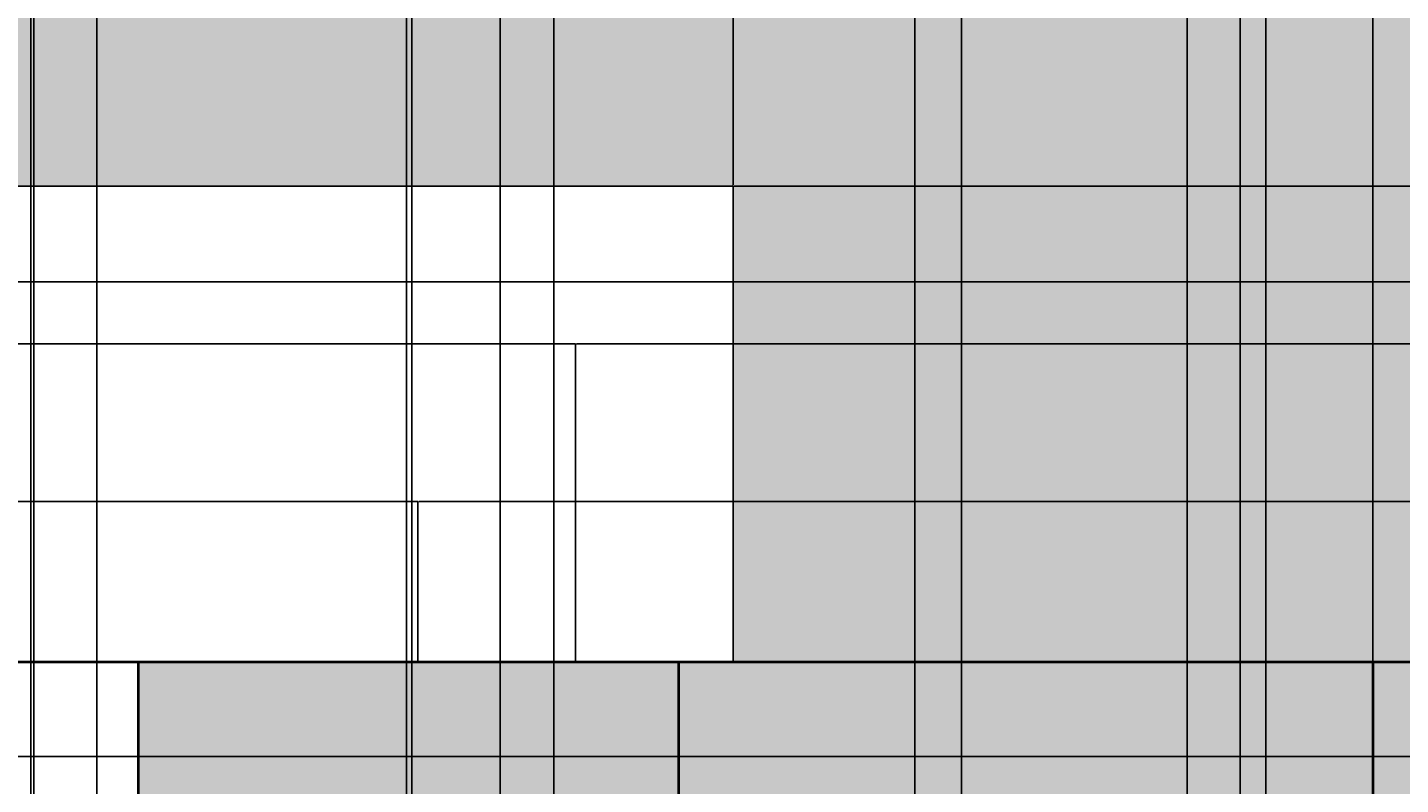
# Model space of a CAD drawing. Units: inches. Extents: x 818 to 1898, y 976 to 2364.
# Tile 66 of 96: x 1173 to 1260, y 2045 to 2093. Entities that reach past the tile are written whole.
import ezdxf

# ---------------------------------------------------------------- set-up
doc = ezdxf.new("R2010")
doc.units = ezdxf.units.IN
doc.header["$LTSCALE"] = 5
doc.header["$MEASUREMENT"] = 0
for name, color, linetype, lineweight in [('A-ANNO-DIMS', 2, 'Continuous', 18), ('A-FLOR-STRS', 7, 'Continuous', 25), ('A-WALL', 7, 'Continuous', 40)]:
    doc.layers.add(name, color=color, linetype=linetype, lineweight=lineweight)
doc.layers.add('A-WALL-PATT', color=251, linetype='Continuous', lineweight=13, true_color=0x636466)
doc.layers.add('L-PLNT-PATT', color=114, linetype='Continuous', lineweight=9, true_color=0x139b48)
doc.styles.get("Standard").update_dxf_attribs({"font": 'arial.ttf'})
doc.dimstyles.get("Standard").update_dxf_attribs({"dimtxt": 0.18, "dimasz": 0.18, "dimexe": 0.18, "dimexo": 0.0625, "dimgap": 0.09, "dimtad": 0, "dimtih": 1, "dimtoh": 1, "dimdec": 4, "dimzin": 0, "dimdsep": 46, "dimtxsty": 'Standard', "dimcen": 0.09, "dimadec": 0, "dimazin": 0, "dimtfac": 1, "dimtdec": 4, "dimtofl": 0, "dimtmove": 0, "dimatfit": 3, "dimfxl": 1, "dimtolj": 1, "dimtzin": 0, "dimarcsym": 0})

# ---------------------------------------------------------------- blocks, each defined once
blk = doc.blocks.new('*D59')
at = {"layer": 'A-ANNO-DIMS', "color": 0, "lineweight": -2, "ltscale": 5, "transparency": 16777216}
for p, q in [((1251.643, 2300.393), (818.026, 2300.393)), ((818.206, 2300.213), (818.206, 1669.95)), ((818.206, 1039.323), (818.206, 1669.586)), ((896.051, 1039.143), (818.026, 1039.143))]:
    blk.add_line(p, q, dxfattribs=at)
at = {"layer": 'A-ANNO-DIMS', "color": 0, "ltscale": 5, "transparency": 16777216}
for points in [[(818.176, 2300.213), (818.236, 2300.213), (818.206, 2300.393)], [(818.176, 1039.323), (818.236, 1039.323), (818.206, 1039.143)]]:
    blk.add_solid(points, dxfattribs=at)
at = {"layer": 'Defpoints', "color": 0, "ltscale": 5, "transparency": 16777216}
for p in [(818.206, 2300.393), (1251.706, 2300.393), (896.114, 1039.143)]:
    blk.add_point(p, dxfattribs=at)
at = {"layer": 'A-ANNO-DIMS', "color": 0, "ltscale": 5, "transparency": 16777216, "insert": (818.206, 1669.768), "char_height": 0.18, "attachment_point": 5}
blk.add_mtext('\\A1;1261.2', dxfattribs=at)
blk = doc.blocks.new('*D61')
at = {"layer": 'A-ANNO-DIMS', "color": 0, "lineweight": -2, "ltscale": 5, "transparency": 16777216}
for p, q in [((1071.725, 1203.027), (1071.725, 2363.873)), ((1071.905, 2363.693), (1250.936, 2363.693)), ((1430.545, 2363.693), (1251.514, 2363.693)), ((1430.725, 1203.027), (1430.725, 2363.873))]:
    blk.add_line(p, q, dxfattribs=at)
at = {"layer": 'A-ANNO-DIMS', "color": 0, "ltscale": 5, "transparency": 16777216}
for points in [[(1071.905, 2363.723), (1071.905, 2363.663), (1071.725, 2363.693)], [(1430.545, 2363.723), (1430.545, 2363.663), (1430.725, 2363.693)]]:
    blk.add_solid(points, dxfattribs=at)
at = {"layer": 'Defpoints', "color": 0, "ltscale": 5, "transparency": 16777216}
for p in [(1430.725, 2363.693), (1071.725, 1202.964), (1430.725, 1202.964)]:
    blk.add_point(p, dxfattribs=at)
at = {"layer": 'A-ANNO-DIMS', "color": 0, "ltscale": 5, "transparency": 16777216, "insert": (1251.225, 2363.693), "char_height": 0.18, "attachment_point": 5}
blk.add_mtext('\\A1;359', dxfattribs=at)
blk = doc.blocks.new('*D64')
at = {"layer": 'A-ANNO-DIMS', "color": 0, "lineweight": -2, "ltscale": 5, "transparency": 16777216}
for p, q in [((1197.725, 1501.141), (1197.725, 2363.873)), ((1197.905, 2363.693), (1313.935, 2363.693)), ((1430.545, 2363.693), (1314.516, 2363.693)), ((1430.725, 1501.141), (1430.725, 2363.873))]:
    blk.add_line(p, q, dxfattribs=at)
at = {"layer": 'A-ANNO-DIMS', "color": 0, "ltscale": 5, "transparency": 16777216}
for points in [[(1197.905, 2363.723), (1197.905, 2363.663), (1197.725, 2363.693)], [(1430.545, 2363.723), (1430.545, 2363.663), (1430.725, 2363.693)]]:
    blk.add_solid(points, dxfattribs=at)
at = {"layer": 'Defpoints', "color": 0, "ltscale": 5, "transparency": 16777216}
for p in [(1430.725, 2363.693), (1197.725, 1501.078), (1430.725, 1501.078)]:
    blk.add_point(p, dxfattribs=at)
at = {"layer": 'A-ANNO-DIMS', "color": 0, "ltscale": 5, "transparency": 16777216, "insert": (1314.225, 2363.693), "char_height": 0.18, "attachment_point": 5}
blk.add_mtext('\\A1;233', dxfattribs=at)
blk = doc.blocks.new('*D82')
at = {"layer": 'A-ANNO-DIMS', "color": 0, "lineweight": -2, "ltscale": 5, "transparency": 16777216}
for p, q in [((1083.725, 1501.141), (1083.725, 2363.873)), ((1083.905, 2363.693), (1140.445, 2363.693)), ((1197.545, 2363.693), (1141.005, 2363.693)), ((1197.725, 1501.141), (1197.725, 2363.873))]:
    blk.add_line(p, q, dxfattribs=at)
at = {"layer": 'A-ANNO-DIMS', "color": 0, "ltscale": 5, "transparency": 16777216}
for points in [[(1083.905, 2363.723), (1083.905, 2363.663), (1083.725, 2363.693)], [(1197.545, 2363.723), (1197.545, 2363.663), (1197.725, 2363.693)]]:
    blk.add_solid(points, dxfattribs=at)
at = {"layer": 'Defpoints', "color": 0, "ltscale": 5, "transparency": 16777216}
for p in [(1197.725, 2363.693), (1083.725, 1501.078), (1197.725, 1501.078)]:
    blk.add_point(p, dxfattribs=at)
at = {"layer": 'A-ANNO-DIMS', "color": 0, "ltscale": 5, "transparency": 16777216, "insert": (1140.725, 2363.693), "char_height": 0.18, "attachment_point": 5}
blk.add_mtext('\\A1;114', dxfattribs=at)
blk = doc.blocks.new('*D83')
at = {"layer": 'A-ANNO-DIMS', "color": 0, "lineweight": -2, "ltscale": 5, "transparency": 16777216}
for p, q in [((1197.725, 1700.141), (1197.725, 2363.873)), ((1197.905, 2363.693), (1228.023, 2363.693)), ((1258.545, 2363.693), (1228.427, 2363.693)), ((1258.725, 1700.141), (1258.725, 2363.873))]:
    blk.add_line(p, q, dxfattribs=at)
at = {"layer": 'A-ANNO-DIMS', "color": 0, "ltscale": 5, "transparency": 16777216}
for points in [[(1197.905, 2363.723), (1197.905, 2363.663), (1197.725, 2363.693)], [(1258.545, 2363.723), (1258.545, 2363.663), (1258.725, 2363.693)]]:
    blk.add_solid(points, dxfattribs=at)
at = {"layer": 'Defpoints', "color": 0, "ltscale": 5, "transparency": 16777216}
for p in [(1258.725, 2363.693), (1197.725, 1700.078), (1258.725, 1700.078)]:
    blk.add_point(p, dxfattribs=at)
at = {"layer": 'A-ANNO-DIMS', "color": 0, "ltscale": 5, "transparency": 16777216, "insert": (1228.225, 2363.693), "char_height": 0.18, "attachment_point": 5}
blk.add_mtext('\\A1;61', dxfattribs=at)
blk = doc.blocks.new('*D85')
at = {"layer": 'A-ANNO-DIMS', "color": 0, "lineweight": -2, "ltscale": 5, "transparency": 16777216}
for p, q in [((1258.788, 2053.078), (1897.916, 2053.078)), ((1897.736, 2052.898), (1897.736, 1876.76)), ((1897.736, 1700.258), (1897.736, 1876.396)), ((1258.788, 1700.078), (1897.916, 1700.078))]:
    blk.add_line(p, q, dxfattribs=at)
at = {"layer": 'A-ANNO-DIMS', "color": 0, "ltscale": 5, "transparency": 16777216}
for points in [[(1897.706, 2052.898), (1897.766, 2052.898), (1897.736, 2053.078)], [(1897.706, 1700.258), (1897.766, 1700.258), (1897.736, 1700.078)]]:
    blk.add_solid(points, dxfattribs=at)
at = {"layer": 'Defpoints', "color": 0, "ltscale": 5, "transparency": 16777216}
for p in [(1258.725, 2053.078), (1897.736, 2053.078), (1258.725, 1700.078)]:
    blk.add_point(p, dxfattribs=at)
at = {"layer": 'A-ANNO-DIMS', "color": 0, "ltscale": 5, "transparency": 16777216, "insert": (1897.736, 1876.578), "char_height": 0.18, "attachment_point": 5}
blk.add_mtext('\\A1;353', dxfattribs=at)
blk = doc.blocks.new('*D86')
at = {"layer": 'A-ANNO-DIMS', "color": 0, "lineweight": -2, "ltscale": 5, "transparency": 16777216}
for p, q in [((1258.725, 2053.141), (1258.725, 2363.873)), ((1258.905, 2363.693), (1486.433, 2363.693)), ((1714.545, 2363.693), (1487.018, 2363.693)), ((1714.725, 2053.141), (1714.725, 2363.873))]:
    blk.add_line(p, q, dxfattribs=at)
at = {"layer": 'A-ANNO-DIMS', "color": 0, "ltscale": 5, "transparency": 16777216}
for points in [[(1258.905, 2363.723), (1258.905, 2363.663), (1258.725, 2363.693)], [(1714.545, 2363.723), (1714.545, 2363.663), (1714.725, 2363.693)]]:
    blk.add_solid(points, dxfattribs=at)
at = {"layer": 'Defpoints', "color": 0, "ltscale": 5, "transparency": 16777216}
for p in [(1714.725, 2363.693), (1258.725, 2053.078), (1714.725, 2053.078)]:
    blk.add_point(p, dxfattribs=at)
at = {"layer": 'A-ANNO-DIMS', "color": 0, "ltscale": 5, "transparency": 16777216, "insert": (1486.725, 2363.693), "char_height": 0.18, "attachment_point": 5}
blk.add_mtext('\\A1;456', dxfattribs=at)
blk = doc.blocks.new('*D94')
at = {"layer": 'A-ANNO-DIMS', "color": 0, "lineweight": -2, "ltscale": 5, "transparency": 16777216}
for p, q in [((1120.762, 1071.118), (1120.762, 2363.873)), ((1120.942, 2363.693), (1146.758, 2363.693)), ((1173.362, 2363.693), (1147.546, 2363.693)), ((1173.542, 1071.118), (1173.542, 2363.873))]:
    blk.add_line(p, q, dxfattribs=at)
at = {"layer": 'A-ANNO-DIMS', "color": 0, "ltscale": 5, "transparency": 16777216}
for points in [[(1120.942, 2363.723), (1120.942, 2363.663), (1120.762, 2363.693)], [(1173.362, 2363.723), (1173.362, 2363.663), (1173.542, 2363.693)]]:
    blk.add_solid(points, dxfattribs=at)
at = {"layer": 'Defpoints', "color": 0, "ltscale": 5, "transparency": 16777216}
for p in [(1173.542, 2363.693), (1120.762, 1071.055), (1173.542, 1071.055)]:
    blk.add_point(p, dxfattribs=at)
at = {"layer": 'A-ANNO-DIMS', "color": 0, "ltscale": 5, "transparency": 16777216, "insert": (1147.152, 2363.693), "char_height": 0.18, "attachment_point": 5}
blk.add_mtext('\\A1;52.78', dxfattribs=at)
blk = doc.blocks.new('*D95')
at = {"layer": 'A-ANNO-DIMS', "color": 0, "lineweight": -2, "ltscale": 5, "transparency": 16777216}
for p, q in [((1173.542, 1071.118), (1173.542, 2363.873)), ((1173.722, 2363.693), (1201.288, 2363.693)), ((1229.467, 2363.693), (1201.901, 2363.693)), ((1229.647, 1071.118), (1229.647, 2363.873))]:
    blk.add_line(p, q, dxfattribs=at)
at = {"layer": 'A-ANNO-DIMS', "color": 0, "ltscale": 5, "transparency": 16777216}
for points in [[(1173.722, 2363.723), (1173.722, 2363.663), (1173.542, 2363.693)], [(1229.467, 2363.723), (1229.467, 2363.663), (1229.647, 2363.693)]]:
    blk.add_solid(points, dxfattribs=at)
at = {"layer": 'Defpoints', "color": 0, "ltscale": 5, "transparency": 16777216}
for p in [(1229.647, 2363.693), (1173.542, 1071.055), (1229.647, 1071.055)]:
    blk.add_point(p, dxfattribs=at)
at = {"layer": 'A-ANNO-DIMS', "color": 0, "ltscale": 5, "transparency": 16777216, "insert": (1201.595, 2363.693), "char_height": 0.18, "attachment_point": 5}
blk.add_mtext('\\A1;56.1', dxfattribs=at)
blk = doc.blocks.new('*D96')
at = {"layer": 'A-ANNO-DIMS', "color": 0, "lineweight": -2, "ltscale": 5, "transparency": 16777216}
for p, q in [((1229.647, 1071.118), (1229.647, 2363.873)), ((1229.827, 2363.693), (1256.516, 2363.693)), ((1283.99, 2363.693), (1257.301, 2363.693)), ((1284.17, 1071.118), (1284.17, 2363.873))]:
    blk.add_line(p, q, dxfattribs=at)
at = {"layer": 'A-ANNO-DIMS', "color": 0, "ltscale": 5, "transparency": 16777216}
for points in [[(1229.827, 2363.723), (1229.827, 2363.663), (1229.647, 2363.693)], [(1283.99, 2363.723), (1283.99, 2363.663), (1284.17, 2363.693)]]:
    blk.add_solid(points, dxfattribs=at)
at = {"layer": 'Defpoints', "color": 0, "ltscale": 5, "transparency": 16777216}
for p in [(1284.17, 2363.693), (1229.647, 1071.055), (1284.17, 1071.055)]:
    blk.add_point(p, dxfattribs=at)
at = {"layer": 'A-ANNO-DIMS', "color": 0, "ltscale": 5, "transparency": 16777216, "insert": (1256.909, 2363.693), "char_height": 0.18, "attachment_point": 5}
blk.add_mtext('\\A1;54.52', dxfattribs=at)
blk = doc.blocks.new('*D109')
at = {"layer": 'A-ANNO-DIMS', "color": 0, "lineweight": -2, "ltscale": 5, "transparency": 16777216}
for p, q in [((1125.917, 1410.117), (1125.917, 2363.873)), ((1126.097, 2363.693), (1164.248, 2363.693)), ((1203.149, 2363.693), (1164.999, 2363.693)), ((1203.329, 1409.911), (1203.329, 2363.873))]:
    blk.add_line(p, q, dxfattribs=at)
at = {"layer": 'A-ANNO-DIMS', "color": 0, "ltscale": 5, "transparency": 16777216}
for points in [[(1126.097, 2363.723), (1126.097, 2363.663), (1125.917, 2363.693)], [(1203.149, 2363.723), (1203.149, 2363.663), (1203.329, 2363.693)]]:
    blk.add_solid(points, dxfattribs=at)
at = {"layer": 'Defpoints', "color": 0, "ltscale": 5, "transparency": 16777216}
for p in [(1203.329, 2363.693), (1125.917, 1410.055), (1203.329, 1409.848)]:
    blk.add_point(p, dxfattribs=at)
at = {"layer": 'A-ANNO-DIMS', "color": 0, "ltscale": 5, "transparency": 16777216, "insert": (1164.623, 2363.693), "char_height": 0.18, "attachment_point": 5}
blk.add_mtext('\\A1;77.41', dxfattribs=at)
blk = doc.blocks.new('*D140')
at = {"layer": 'A-ANNO-DIMS', "color": 0, "lineweight": -2, "ltscale": 5, "transparency": 16777216}
for p, q in [((1083.725, 2053.141), (1083.725, 2363.873)), ((1083.905, 2363.693), (1150.463, 2363.693)), ((1217.931, 2363.693), (1151.374, 2363.693)), ((1218.111, 2083.325), (1218.111, 2363.873))]:
    blk.add_line(p, q, dxfattribs=at)
at = {"layer": 'A-ANNO-DIMS', "color": 0, "ltscale": 5, "transparency": 16777216}
for points in [[(1083.905, 2363.723), (1083.905, 2363.663), (1083.725, 2363.693)], [(1217.931, 2363.723), (1217.931, 2363.663), (1218.111, 2363.693)]]:
    blk.add_solid(points, dxfattribs=at)
at = {"layer": 'Defpoints', "color": 0, "ltscale": 5, "transparency": 16777216}
for p in [(1218.111, 2363.693), (1218.111, 2083.262), (1083.725, 2053.078)]:
    blk.add_point(p, dxfattribs=at)
at = {"layer": 'A-ANNO-DIMS', "color": 0, "ltscale": 5, "transparency": 16777216, "insert": (1150.918, 2363.693), "char_height": 0.18, "attachment_point": 5}
blk.add_mtext('\\A1;134.39', dxfattribs=at)
blk = doc.blocks.new('*D141')
at = {"layer": 'A-ANNO-DIMS', "color": 0, "lineweight": -2, "ltscale": 5, "transparency": 16777216}
for p, q in [((1218.174, 2083.262), (1897.916, 2083.262)), ((1897.736, 2083.082), (1897.736, 2073.444)), ((1897.736, 2063.442), (1897.736, 2073.08)), ((1198.174, 2063.262), (1897.916, 2063.262))]:
    blk.add_line(p, q, dxfattribs=at)
at = {"layer": 'A-ANNO-DIMS', "color": 0, "ltscale": 5, "transparency": 16777216}
for points in [[(1897.706, 2083.082), (1897.766, 2083.082), (1897.736, 2083.262)], [(1897.706, 2063.442), (1897.766, 2063.442), (1897.736, 2063.262)]]:
    blk.add_solid(points, dxfattribs=at)
at = {"layer": 'Defpoints', "color": 0, "ltscale": 5, "transparency": 16777216}
for p in [(1218.111, 2083.262), (1198.111, 2063.262), (1897.736, 2063.262)]:
    blk.add_point(p, dxfattribs=at)
at = {"layer": 'A-ANNO-DIMS', "color": 0, "ltscale": 5, "transparency": 16777216, "insert": (1897.736, 2073.262), "char_height": 0.18, "attachment_point": 5}
blk.add_mtext('\\A1;20', dxfattribs=at)
blk = doc.blocks.new('*D142')
at = {"layer": 'A-ANNO-DIMS', "color": 0, "lineweight": -2, "ltscale": 5, "transparency": 16777216}
for p, q in [((1208.174, 2073.262), (1897.916, 2073.262)), ((1897.736, 2073.082), (1897.736, 2068.444)), ((1897.736, 2063.442), (1897.736, 2068.08)), ((1198.174, 2063.262), (1897.916, 2063.262))]:
    blk.add_line(p, q, dxfattribs=at)
at = {"layer": 'A-ANNO-DIMS', "color": 0, "ltscale": 5, "transparency": 16777216}
for points in [[(1897.706, 2073.082), (1897.766, 2073.082), (1897.736, 2073.262)], [(1897.706, 2063.442), (1897.766, 2063.442), (1897.736, 2063.262)]]:
    blk.add_solid(points, dxfattribs=at)
at = {"layer": 'Defpoints', "color": 0, "ltscale": 5, "transparency": 16777216}
for p in [(1208.111, 2073.262), (1897.736, 2073.262), (1198.111, 2063.262)]:
    blk.add_point(p, dxfattribs=at)
at = {"layer": 'A-ANNO-DIMS', "color": 0, "ltscale": 5, "transparency": 16777216, "insert": (1897.736, 2068.262), "char_height": 0.18, "attachment_point": 5}
blk.add_mtext('\\A1;10', dxfattribs=at)
blk = doc.blocks.new('*D145')
at = {"layer": 'A-ANNO-DIMS', "color": 0, "lineweight": -2, "ltscale": 5, "transparency": 16777216}
for p, q in [((1197.393, 2122.314), (1197.393, 975.663)), ((1232.609, 2122.314), (1232.609, 975.663)), ((1197.573, 975.843), (1214.608, 975.843)), ((1232.429, 975.843), (1215.394, 975.843))]:
    blk.add_line(p, q, dxfattribs=at)
at = {"layer": 'A-ANNO-DIMS', "color": 0, "ltscale": 5, "transparency": 16777216}
for points in [[(1197.573, 975.873), (1197.573, 975.813), (1197.393, 975.843)], [(1232.429, 975.873), (1232.429, 975.813), (1232.609, 975.843)]]:
    blk.add_solid(points, dxfattribs=at)
at = {"layer": 'Defpoints', "color": 0, "ltscale": 5, "transparency": 16777216}
for p in [(1197.393, 2122.377), (1232.609, 2122.377), (1232.609, 975.843)]:
    blk.add_point(p, dxfattribs=at)
at = {"layer": 'A-ANNO-DIMS', "color": 0, "ltscale": 5, "transparency": 16777216, "insert": (1215.001, 975.843), "char_height": 0.18, "attachment_point": 5}
blk.add_mtext('\\A1;35.22', dxfattribs=at)
blk = doc.blocks.new('*D146')
at = {"layer": 'A-ANNO-DIMS', "color": 0, "lineweight": -2, "ltscale": 5, "transparency": 16777216}
for p, q in [((1197.33, 2122.377), (818.026, 2122.377)), ((818.206, 2122.197), (818.206, 2087.909)), ((818.206, 2053.258), (818.206, 2087.546)), ((1083.663, 2053.078), (818.026, 2053.078))]:
    blk.add_line(p, q, dxfattribs=at)
at = {"layer": 'A-ANNO-DIMS', "color": 0, "ltscale": 5, "transparency": 16777216}
for points in [[(818.176, 2122.197), (818.236, 2122.197), (818.206, 2122.377)], [(818.176, 2053.258), (818.236, 2053.258), (818.206, 2053.078)]]:
    blk.add_solid(points, dxfattribs=at)
at = {"layer": 'Defpoints', "color": 0, "ltscale": 5, "transparency": 16777216}
for p in [(1197.393, 2122.377), (818.206, 2053.078), (1083.725, 2053.078)]:
    blk.add_point(p, dxfattribs=at)
at = {"layer": 'A-ANNO-DIMS', "color": 0, "ltscale": 5, "transparency": 16777216, "insert": (818.206, 2087.727), "char_height": 0.18, "attachment_point": 5}
blk.add_mtext('\\A1;69.3', dxfattribs=at)
blk = doc.blocks.new('*D158')
at = {"layer": 'A-ANNO-DIMS', "color": 0, "lineweight": -2, "ltscale": 5, "transparency": 16777216}
for p, q in [((1173.725, 1590.821), (1173.725, 2363.873)), ((1173.905, 2363.693), (1175.573, 2363.693)), ((1177.545, 2363.693), (1175.877, 2363.693)), ((1177.725, 1586.821), (1177.725, 2363.873))]:
    blk.add_line(p, q, dxfattribs=at)
at = {"layer": 'A-ANNO-DIMS', "color": 0, "ltscale": 5, "transparency": 16777216}
for points in [[(1173.905, 2363.723), (1173.905, 2363.663), (1173.725, 2363.693)], [(1177.545, 2363.723), (1177.545, 2363.663), (1177.725, 2363.693)]]:
    blk.add_solid(points, dxfattribs=at)
at = {"layer": 'Defpoints', "color": 0, "ltscale": 5, "transparency": 16777216}
for p in [(1177.725, 2363.693), (1173.725, 1590.758), (1177.725, 1586.758)]:
    blk.add_point(p, dxfattribs=at)
at = {"layer": 'A-ANNO-DIMS', "color": 0, "ltscale": 5, "transparency": 16777216, "insert": (1175.725, 2363.693), "char_height": 0.18, "attachment_point": 5}
blk.add_mtext('\\A1;4', dxfattribs=at)
blk = doc.blocks.new('*D257')
at = {"layer": 'A-ANNO-DIMS', "color": 0, "lineweight": -2, "ltscale": 5, "transparency": 16777216}
for p, q in [((1399.573, 2077.188), (818.026, 2077.188)), ((818.206, 2077.008), (818.206, 2065.314)), ((818.206, 2053.258), (818.206, 2064.953)), ((1399.573, 2053.078), (818.026, 2053.078))]:
    blk.add_line(p, q, dxfattribs=at)
at = {"layer": 'A-ANNO-DIMS', "color": 0, "ltscale": 5, "transparency": 16777216}
for points in [[(818.176, 2077.008), (818.236, 2077.008), (818.206, 2077.188)], [(818.176, 2053.258), (818.236, 2053.258), (818.206, 2053.078)]]:
    blk.add_solid(points, dxfattribs=at)
at = {"layer": 'Defpoints', "color": 0, "ltscale": 5, "transparency": 16777216}
for p in [(818.206, 2077.188), (1399.636, 2077.188), (1399.636, 2053.078)]:
    blk.add_point(p, dxfattribs=at)
at = {"layer": 'A-ANNO-DIMS', "color": 0, "ltscale": 5, "transparency": 16777216, "insert": (818.206, 2065.133), "char_height": 0.18, "attachment_point": 5}
blk.add_mtext('\\A1;24.11', dxfattribs=at)
blk = doc.blocks.new('*D266')
at = {"layer": 'A-ANNO-DIMS', "color": 0, "lineweight": -2, "ltscale": 5, "transparency": 16777216}
for p, q in [((1780.439, 2053.078), (818.026, 2053.078)), ((818.206, 2052.898), (818.206, 2050.26)), ((818.206, 2047.258), (818.206, 2049.896)), ((1780.439, 2047.078), (818.026, 2047.078))]:
    blk.add_line(p, q, dxfattribs=at)
at = {"layer": 'A-ANNO-DIMS', "color": 0, "ltscale": 5, "transparency": 16777216}
for points in [[(818.176, 2052.898), (818.236, 2052.898), (818.206, 2053.078)], [(818.176, 2047.258), (818.236, 2047.258), (818.206, 2047.078)]]:
    blk.add_solid(points, dxfattribs=at)
at = {"layer": 'Defpoints', "color": 0, "ltscale": 5, "transparency": 16777216}
for p in [(1780.502, 2053.078), (818.206, 2047.078), (1780.502, 2047.078)]:
    blk.add_point(p, dxfattribs=at)
at = {"layer": 'A-ANNO-DIMS', "color": 0, "ltscale": 5, "transparency": 16777216, "insert": (818.206, 2050.078), "char_height": 0.18, "attachment_point": 5}
blk.add_mtext('\\A1;6', dxfattribs=at)
blk = doc.blocks.new('*D269')
at = {"layer": 'A-ANNO-DIMS', "color": 0, "lineweight": -2, "ltscale": 5, "transparency": 16777216}
for p, q in [((1246.938, 1534.141), (1246.938, 2363.873)), ((1247.118, 2363.693), (1293.706, 2363.693)), ((1341.079, 2363.693), (1294.491, 2363.693)), ((1341.259, 1534.141), (1341.259, 2363.873))]:
    blk.add_line(p, q, dxfattribs=at)
at = {"layer": 'A-ANNO-DIMS', "color": 0, "ltscale": 5, "transparency": 16777216}
for points in [[(1247.118, 2363.723), (1247.118, 2363.663), (1246.938, 2363.693)], [(1341.079, 2363.723), (1341.079, 2363.663), (1341.259, 2363.693)]]:
    blk.add_solid(points, dxfattribs=at)
at = {"layer": 'Defpoints', "color": 0, "ltscale": 5, "transparency": 16777216}
for p in [(1341.259, 2363.693), (1246.938, 1534.078), (1341.259, 1534.078)]:
    blk.add_point(p, dxfattribs=at)
at = {"layer": 'A-ANNO-DIMS', "color": 0, "ltscale": 5, "transparency": 16777216, "insert": (1294.099, 2363.693), "char_height": 0.18, "attachment_point": 5}
blk.add_mtext('\\A1;94.32', dxfattribs=at)
blk = doc.blocks.new('*D271')
at = {"layer": 'A-ANNO-DIMS', "color": 0, "lineweight": -2, "ltscale": 5, "transparency": 16777216}
for p, q in [((1206.725, 1510.141), (1206.725, 2363.873)), ((1206.905, 2363.693), (1226.451, 2363.693)), ((1246.758, 2363.693), (1227.211, 2363.693)), ((1246.938, 1510.141), (1246.938, 2363.873))]:
    blk.add_line(p, q, dxfattribs=at)
at = {"layer": 'A-ANNO-DIMS', "color": 0, "ltscale": 5, "transparency": 16777216}
for points in [[(1206.905, 2363.723), (1206.905, 2363.663), (1206.725, 2363.693)], [(1246.758, 2363.723), (1246.758, 2363.663), (1246.938, 2363.693)]]:
    blk.add_solid(points, dxfattribs=at)
at = {"layer": 'Defpoints', "color": 0, "ltscale": 5, "transparency": 16777216}
for p in [(1246.938, 2363.693), (1206.725, 1510.078), (1246.938, 1510.078)]:
    blk.add_point(p, dxfattribs=at)
at = {"layer": 'A-ANNO-DIMS', "color": 0, "ltscale": 5, "transparency": 16777216, "insert": (1226.831, 2363.693), "char_height": 0.18, "attachment_point": 5}
blk.add_mtext('\\A1;40.21', dxfattribs=at)
blk = doc.blocks.new('*D276')
at = {"layer": 'A-ANNO-DIMS', "color": 0, "lineweight": -2, "ltscale": 5, "transparency": 16777216}
for p, q in [((1206.725, 1687.141), (1206.725, 2363.873)), ((1206.905, 2363.693), (1228.949, 2363.693)), ((1251.753, 2363.693), (1229.709, 2363.693)), ((1251.933, 1681.439), (1251.933, 2363.873))]:
    blk.add_line(p, q, dxfattribs=at)
at = {"layer": 'A-ANNO-DIMS', "color": 0, "ltscale": 5, "transparency": 16777216}
for points in [[(1206.905, 2363.723), (1206.905, 2363.663), (1206.725, 2363.693)], [(1251.753, 2363.723), (1251.753, 2363.663), (1251.933, 2363.693)]]:
    blk.add_solid(points, dxfattribs=at)
at = {"layer": 'Defpoints', "color": 0, "ltscale": 5, "transparency": 16777216}
for p in [(1251.933, 2363.693), (1206.725, 1687.078), (1251.933, 1681.376)]:
    blk.add_point(p, dxfattribs=at)
at = {"layer": 'A-ANNO-DIMS', "color": 0, "ltscale": 5, "transparency": 16777216, "insert": (1229.329, 2363.693), "char_height": 0.18, "attachment_point": 5}
blk.add_mtext('\\A1;45.21', dxfattribs=at)
blk = doc.blocks.new('*D281')
at = {"layer": 'A-ANNO-DIMS', "color": 0, "lineweight": -2, "ltscale": 5, "transparency": 16777216}
for p, q in [((1250.303, 1913.703), (1250.303, 2363.873)), ((1250.483, 2363.693), (1420.121, 2363.693)), ((1590.545, 2363.693), (1420.907, 2363.693)), ((1590.725, 2011.141), (1590.725, 2363.873))]:
    blk.add_line(p, q, dxfattribs=at)
at = {"layer": 'A-ANNO-DIMS', "color": 0, "ltscale": 5, "transparency": 16777216}
for points in [[(1250.483, 2363.723), (1250.483, 2363.663), (1250.303, 2363.693)], [(1590.545, 2363.723), (1590.545, 2363.663), (1590.725, 2363.693)]]:
    blk.add_solid(points, dxfattribs=at)
at = {"layer": 'Defpoints', "color": 0, "ltscale": 5, "transparency": 16777216}
for p in [(1590.725, 2363.693), (1590.725, 2011.078), (1250.303, 1913.64)]:
    blk.add_point(p, dxfattribs=at)
at = {"layer": 'A-ANNO-DIMS', "color": 0, "ltscale": 5, "transparency": 16777216, "insert": (1420.514, 2363.693), "char_height": 0.18, "attachment_point": 5}
blk.add_mtext('\\A1;340.4', dxfattribs=at)

msp = doc.modelspace()

# ---------------------------------------------------------------- hatches: boundary and pattern name
at = {"layer": 'A-WALL-PATT', "ltscale": 5}
h = msp.add_hatch(color=256, dxfattribs=at)
h.dxf.hatch_style = 1
h.paths.add_polyline_path([(1267.7252, 1928.9218), (1258.7251, 1928.9218), (1258.7251, 1913.6401), (1250.3029, 1913.6401), (1250.3029, 1878.3919), (1258.7251, 1878.3919), (1258.7251, 1862.9652), (1267.7252, 1862.9652)])
h.paths.add_polyline_path([(1267.7252, 1814.9652), (1258.7251, 1814.9652), (1258.7251, 1755.3321), (1267.7252, 1755.3321)])
h.paths.add_polyline_path([(1463.7252, 1696.0782), (1267.7252, 1696.0782), (1267.7252, 1707.3321), (1258.7251, 1707.3321), (1258.7251, 1700.0782), (1251.9333, 1700.0782), (1251.9333, 1687.0782), (1463.7252, 1687.0782)])
h.paths.add_polyline_path([(1714.7251, 1717.3178), (1705.7252, 1717.3178), (1705.7252, 1696.0782), (1599.7252, 1696.0782), (1599.7252, 1790.0782), (1705.7252, 1790.0782), (1705.7252, 1785.6125), (1714.7251, 1785.6125), (1714.7251, 1827.2125), (1705.7252, 1827.2125), (1705.7252, 1802.0782), (1599.7252, 1802.0782), (1599.7252, 1867.0782), (1705.7252, 1867.0782), (1705.7252, 1857.2125), (1714.7251, 1857.2125), (1714.7251, 1930.0316), (1741.8409, 1930.0316), (1741.8409, 1935.0316), (1714.7251, 1935.0316), (1714.7251, 1957.0338), (1741.8409, 1957.0338), (1741.8409, 1962.0338), (1714.7251, 1962.0338), (1705.7252, 1962.0338), (1705.7252, 1948.0782), (1599.7252, 1948.0782), (1599.7252, 1981.0782), (1590.7251, 1981.0782), (1590.7251, 1941.0782), (1620.7252, 1941.0782), (1705.7252, 1941.0782), (1705.7252, 1876.0782), (1599.7252, 1876.0782), (1599.7252, 1911.0782), (1590.7251, 1911.0782), (1590.7251, 1876.0782), (1429.2252, 1876.0782), (1429.2252, 1867.0782), (1511.7252, 1867.0782), (1528.593, 1867.0782), (1595.7252, 1867.0782), (1595.7252, 1773.0782), (1520.7252, 1773.0782), (1520.7252, 1837.5823), (1532.593, 1837.5823), (1532.593, 1867.0782), (1528.593, 1867.0782), (1528.593, 1841.5823), (1511.7252, 1841.5823), (1511.7252, 1744.9714), (1520.7252, 1744.9714), (1520.7252, 1761.0782), (1595.7252, 1761.0782), (1595.7252, 1696.0782), (1520.7252, 1696.0782), (1520.7252, 1716.0454), (1511.7252, 1716.0454), (1511.7252, 1696.0782), (1511.7252, 1687.0782), (1714.7251, 1687.0782)])
h.paths.add_polyline_path([(1714.7251, 2053.0782), (1714.7251, 2081.1881), (1709.7252, 2081.1881), (1709.7252, 2053.0782), (1681.6446, 2053.0782), (1681.6446, 2081.1881), (1676.6446, 2081.1881), (1676.6446, 2053.0782), (1538.5155, 2053.0782), (1538.5155, 2044.0782), (1590.7251, 2044.0782), (1590.7251, 2011.0782), (1599.7252, 2011.0782), (1599.7252, 2044.0782), (1705.7252, 2044.0782), (1705.7252, 2014.5114), (1714.7251, 2014.5114)])
h.paths.add_polyline_path([(1485.1216, 2053.0782), (1422.02, 2053.0782), (1422.02, 2081.1881), (1413.02, 2081.1881), (1413.02, 2053.0782), (1399.6356, 2053.0782), (1399.6356, 2081.1881), (1390.6356, 2081.1881), (1390.6356, 2053.0782), (1388.0315, 2053.0782), (1388.0315, 2044.0782), (1416.2743, 2044.0782), (1485.1216, 2044.0782)])
h.paths.add_polyline_path([(1330.305, 2053.0782), (1258.7251, 2053.0782), (1258.7251, 2019.2871), (1267.7252, 2019.2871), (1267.7252, 2044.0782), (1330.305, 2044.0782)])
h.paths.add_polyline_path([(1258.7251, 2053.0782), (1214.6577, 2053.0782), (1214.6577, 2044.0782), (1258.7251, 2044.0782)])
h.paths.add_polyline_path([(1214.6577, 2053.0782), (1180.349, 2053.0782), (1180.349, 2044.0782), (1214.6577, 2044.0782)])
h.paths.add_polyline_path([(1714.7251, 1639.5782), (1741.8409, 1639.5782), (1741.8409, 1643.5782), (1714.7251, 1643.5782), (1714.7251, 1649.9029), (1705.7252, 1649.9029), (1705.7252, 1600.0782), (1477.7252, 1600.0782), (1477.7252, 1591.0782), (1520.7252, 1591.0782), (1616.7252, 1591.0782), (1616.7252, 1416.6857), (1622.7252, 1416.6857), (1622.7252, 1463.0782), (1624.7252, 1463.0782), (1624.7252, 1467.0782), (1622.7252, 1467.0782), (1622.7252, 1591.0782), (1705.7252, 1591.0782), (1705.7252, 1545.0782), (1714.7251, 1545.0782), (1741.8409, 1545.0782), (1741.8409, 1549.0782), (1714.7251, 1549.0782), (1714.7251, 1593.9175), (1737.8409, 1593.9175), (1737.8409, 1597.9175), (1714.7251, 1597.9175)])
h.paths.add_polyline_path([(1674.9024, 2060.7419), (1714.7045, 2060.7419), (1714.7045, 2073.1061), (1674.9024, 2073.1061)], flags=25)
h.paths.add_polyline_path([(1394.5468, 2061.6618), (1422.2344, 2061.6618), (1422.2344, 2074.0261), (1394.5468, 2074.0261)], flags=24)
at = {"layer": 'L-PLNT-PATT', "ltscale": 5}
h = msp.add_hatch(color=256, dxfattribs=at)
h.dxf.hatch_style = 1
h.paths.add_polyline_path([(1789.7173, 2205.9709), (1083.7251, 2205.9709), (1083.7251, 2083.2623), (1218.1114, 2083.2623), (1218.1114, 2053.0782), (1390.6356, 2053.0782), (1390.6356, 2081.1881), (1399.6356, 2081.1881), (1413.02, 2081.1881), (1422.02, 2081.1881), (1422.02, 2053.0782), (1676.6446, 2053.0782), (1676.6446, 2081.1881), (1714.7251, 2081.1881), (1714.7251, 2081.6235), (1789.7173, 2081.6235)])
h.paths.add_polyline_path([(1388.6037, 2145.2461), (1388.6037, 2122.3767), (1373.4756, 2122.3767), (1373.4756, 2145.2461)], flags=16)
h.paths.add_polyline_path([(1408.6922, 2145.2461), (1423.8203, 2145.2461), (1423.8203, 2122.3767), (1408.6922, 2122.3767)], flags=16)
h.paths.add_polyline_path([(1353.3871, 2155.7839), (1353.3871, 2122.3767), (1338.259, 2122.3767), (1338.259, 2155.7839)], flags=16)
h.paths.add_polyline_path([(1443.9089, 2158.4222), (1459.037, 2158.4222), (1459.037, 2122.3767), (1443.9089, 2122.3767)], flags=16)
h.paths.add_polyline_path([(1318.1705, 2145.2461), (1318.1705, 2122.3767), (1303.0424, 2122.3767), (1303.0424, 2145.2461)], flags=16)
h.paths.add_polyline_path([(1479.1255, 2145.2461), (1494.2536, 2145.2461), (1494.2536, 2122.3767), (1479.1255, 2122.3767)], flags=16)
h.paths.add_polyline_path([(1282.9539, 2145.2461), (1282.9539, 2122.3767), (1267.8258, 2122.3767), (1267.8258, 2145.2461)], flags=16)
h.paths.add_polyline_path([(1514.3421, 2145.2461), (1529.4702, 2145.2461), (1529.4702, 2122.3767), (1514.3421, 2122.3767)], flags=16)
h.paths.add_polyline_path([(1247.7373, 2159.4296), (1247.7373, 2122.3767), (1232.6091, 2122.3767), (1232.6091, 2159.4296)], flags=16)
h.paths.add_polyline_path([(1549.5587, 2156.9246), (1564.6868, 2156.9246), (1564.6868, 2122.3767), (1549.5587, 2122.3767)], flags=16)
h.paths.add_polyline_path([(1212.5206, 2145.2461), (1212.5206, 2122.3767), (1197.3925, 2122.3767), (1197.3925, 2145.2461)], flags=16)
h.paths.add_polyline_path([(1584.7753, 2145.2461), (1599.9034, 2145.2461), (1599.9034, 2122.3767), (1584.7753, 2122.3767)], flags=16)
h.paths.add_polyline_path([(1185.1073, 2104.7786), (1190.6407, 2104.7786), (1185.1073, 2098.2505), (1179.5738, 2104.7786)], flags=16)
h.paths.add_polyline_path([(1619.9919, 2145.2461), (1635.1201, 2145.2461), (1635.1201, 2122.3767), (1619.9919, 2122.3767)], flags=16)
h.paths.add_polyline_path([(1655.2086, 2156.1761), (1670.3367, 2156.1761), (1670.3367, 2122.3767), (1655.2086, 2122.3767)], flags=16)
h.paths.add_polyline_path([(1686.5992, 2145.2461), (1701.7273, 2145.2461), (1701.7273, 2122.3767), (1686.5992, 2122.3767)], flags=16)
h.paths.add_polyline_path([(1715.7616, 2145.2461), (1730.8897, 2145.2461), (1730.8897, 2122.3767), (1715.7616, 2122.3767)], flags=16)
h.paths.add_polyline_path([(1753.1652, 2145.2461), (1776.3312, 2145.2461), (1776.3312, 2115.6891), (1753.1652, 2115.6891)], flags=16)
h.paths.add_polyline_path([(1191.4331, 2146.5159), (1176.7891, 2146.5159), (1176.7891, 2134.1516), (1191.4331, 2134.1516)], flags=24)

# ---------------------------------------------------------------- linework, layer by layer
at = {"layer": 'A-FLOR-STRS', "ltscale": 5}
for p, q in [((1218.1114, 2083.2623), (1083.7251, 2083.2623)), ((1218.1114, 2053.0782), (1218.1114, 2083.2623)), ((1208.1114, 2073.2623), (1083.7251, 2073.2623)), ((1208.1114, 2053.0782), (1208.1114, 2073.2623)), ((1198.1114, 2063.2623), (1083.7251, 2063.2623)), ((1198.1114, 2053.0782), (1198.1114, 2063.2623)), ((1083.7251, 2053.0782), (1198.1114, 2053.0782))]:
    msp.add_line(p, q, dxfattribs=at)
at = {"layer": 'A-WALL'}
for p, q in [((1083.7251, 2053.0782), (1390.6356, 2053.0782)), ((1258.7251, 2053.0782), (1258.7251, 1913.6401))]:
    msp.add_line(p, q, dxfattribs=at)
at = {"layer": 'A-WALL', "ltscale": 5}
for p, q in [((1180.349, 2053.0782), (1180.349, 2044.0782)), ((1214.6577, 2053.0782), (1214.6577, 2044.0782))]:
    msp.add_line(p, q, dxfattribs=at)

# ---------------------------------------------------------------- dimensions: what is measured, and where the dimension line sits
at = {"layer": 'A-ANNO-DIMS', "ltscale": 5}
for base, p1, p2, override, picture, middle in [((1430.7251, 2363.6929), (1071.7251, 1202.9642), (1430.7251, 1202.9642), {"dimdec": 0, "dimlfac": 1, "dimrnd": 0, "dimzin": 0, "dimdsep": 46, "dimlunit": 2}, '*D61', (1251.2251, 2363.6929)), ((1197.7251, 2363.6929), (1083.7251, 1501.0782), (1197.7251, 1501.0782), {"dimdec": 0, "dimlfac": 1, "dimrnd": 0, "dimzin": 0, "dimdsep": 46, "dimlunit": 2}, '*D82', (1140.7251, 2363.6929)), ((1218.1114, 2363.6929), (1083.7251, 2053.0782), (1218.1114, 2083.2623), {"dimdec": 2, "dimlfac": 1, "dimrnd": 0, "dimzin": 0, "dimdsep": 46, "dimlunit": 2}, '*D140', (1150.9183, 2363.6929)), ((1173.5418, 2363.6929), (1120.7618, 1071.0552), (1173.5418, 1071.0552), {"dimdec": 2, "dimlfac": 1, "dimrnd": 0, "dimzin": 0, "dimdsep": 46, "dimlunit": 2}, '*D94', (1147.1518, 2363.6929)), ((1203.3292, 2363.6929), (1125.9172, 1410.0547), (1203.3292, 1409.8484), {"dimdec": 2, "dimlfac": 1, "dimrnd": 0, "dimzin": 0, "dimdsep": 46, "dimlunit": 2}, '*D109', (1164.6232, 2363.6929)), ((1229.6474, 2363.6929), (1173.5418, 1071.0552), (1229.6474, 1071.0552), {"dimdec": 1, "dimlfac": 1, "dimrnd": 0, "dimzin": 0, "dimdsep": 46, "dimlunit": 2}, '*D95', (1201.5946, 2363.6929)), ((1177.7251, 2363.6929), (1173.7251, 1590.7585), (1177.7251, 1586.7585), {"dimdec": 0, "dimlfac": 1, "dimrnd": 0, "dimzin": 0, "dimdsep": 46, "dimlunit": 2}, '*D158', (1175.7251, 2363.6929)), ((1430.7251, 2363.6929), (1197.7251, 1501.0782), (1430.7251, 1501.0782), {"dimdec": 0, "dimlfac": 1, "dimrnd": 0, "dimzin": 0, "dimdsep": 46, "dimlunit": 2}, '*D64', (1314.2251, 2363.6929)), ((1258.7251, 2363.6929), (1197.7251, 1700.0782), (1258.7251, 1700.0782), {"dimdec": 0, "dimlfac": 1, "dimrnd": 0, "dimzin": 0, "dimdsep": 46, "dimlunit": 2}, '*D83', (1228.2251, 2363.6929)), ((1246.9377, 2363.6929), (1206.7251, 1510.0782), (1246.9377, 1510.0782), {"dimdec": 2, "dimlfac": 1, "dimrnd": 0, "dimzin": 0, "dimdsep": 46, "dimlunit": 2}, '*D271', (1226.8314, 2363.6929)), ((1251.9333, 2363.6929), (1206.7251, 1687.0782), (1251.9333, 1681.3763), {"dimdec": 2, "dimlfac": 1, "dimrnd": 0, "dimzin": 0, "dimdsep": 46, "dimlunit": 2}, '*D276', (1229.3292, 2363.6929)), ((1284.1697, 2363.6929), (1229.6474, 1071.0552), (1284.1697, 1071.0552), {"dimdec": 2, "dimlfac": 1, "dimrnd": 0, "dimzin": 0, "dimdsep": 46, "dimlunit": 2}, '*D96', (1256.9085, 2363.6929)), ((1341.2593, 2363.6929), (1246.9377, 1534.0782), (1341.2593, 1534.0782), {"dimdec": 2, "dimlfac": 1, "dimrnd": 0, "dimzin": 0, "dimdsep": 46, "dimlunit": 2}, '*D269', (1294.0985, 2363.6929)), ((1590.7251, 2363.6929), (1250.3029, 1913.6401), (1590.7251, 2011.0782), {"dimdec": 1, "dimlfac": 1, "dimrnd": 0, "dimzin": 0, "dimdsep": 46, "dimlunit": 2}, '*D281', (1420.514, 2363.6929)), ((1714.7251, 2363.6929), (1258.7251, 2053.0782), (1714.7251, 2053.0782), {"dimdec": 0, "dimlfac": 1, "dimrnd": 0, "dimzin": 0, "dimdsep": 46, "dimlunit": 2}, '*D86', (1486.7251, 2363.6929)), ((1232.6091, 975.8433), (1197.3925, 2122.3767), (1232.6091, 2122.3767), {"dimdec": 2, "dimlfac": 1, "dimrnd": 0, "dimzin": 0, "dimdsep": 46, "dimlunit": 2}, '*D145', (1215.0008, 975.8433))]:
    dim = msp.add_linear_dim(base=base, p1=p1, p2=p2, dimstyle='Standard', override=override, dxfattribs=at)
    dim.commit()
    dim.dimension.update_dxf_attribs({"geometry": picture, "text_midpoint": middle})
for base, p1, p2, override, picture, middle in [((818.2059, 2300.3929), (896.1138, 1039.1433), (1251.7057, 2300.3929), {"dimdec": 1, "dimlfac": 1, "dimrnd": 0, "dimzin": 0, "dimdsep": 46, "dimlunit": 2}, '*D59', (818.2059, 1669.7681)), ((818.2059, 2053.0782), (1197.3925, 2122.3767), (1083.7251, 2053.0782), {"dimdec": 1, "dimlfac": 1, "dimrnd": 0, "dimzin": 0, "dimdsep": 46, "dimlunit": 2}, '*D146', (818.2059, 2087.7275)), ((1897.736, 2063.2623), (1218.1114, 2083.2623), (1198.1114, 2063.2623), {"dimdec": 0, "dimlfac": 1, "dimrnd": 0, "dimzin": 0, "dimdsep": 46, "dimlunit": 2}, '*D141', (1897.736, 2073.2623)), ((818.2059, 2077.1881), (1399.6356, 2053.0782), (1399.6356, 2077.1881), {"dimdec": 2, "dimlfac": 1, "dimrnd": 0, "dimzin": 0, "dimdsep": 46, "dimlunit": 2}, '*D257', (818.2059, 2065.1332)), ((1897.736, 2073.2623), (1198.1114, 2063.2623), (1208.1114, 2073.2623), {"dimdec": 0, "dimlfac": 1, "dimrnd": 0, "dimzin": 0, "dimdsep": 46, "dimlunit": 2}, '*D142', (1897.736, 2068.2623)), ((818.2059, 2047.0782), (1780.5019, 2053.0782), (1780.5019, 2047.0782), {"dimdec": 0, "dimlfac": 1, "dimrnd": 0, "dimzin": 0, "dimdsep": 46, "dimlunit": 2}, '*D266', (818.2059, 2050.0782)), ((1897.736, 2053.0782), (1258.7251, 1700.0782), (1258.7251, 2053.0782), {"dimdec": 0, "dimlfac": 1, "dimrnd": 0, "dimzin": 0, "dimdsep": 46, "dimlunit": 2}, '*D85', (1897.736, 1876.5782))]:
    dim = msp.add_linear_dim(base=base, p1=p1, p2=p2, angle=90, dimstyle='Standard', override=override, dxfattribs=at)
    dim.commit()
    dim.dimension.update_dxf_attribs({"geometry": picture, "text_midpoint": middle})

doc.saveas('drawing.dxf')
